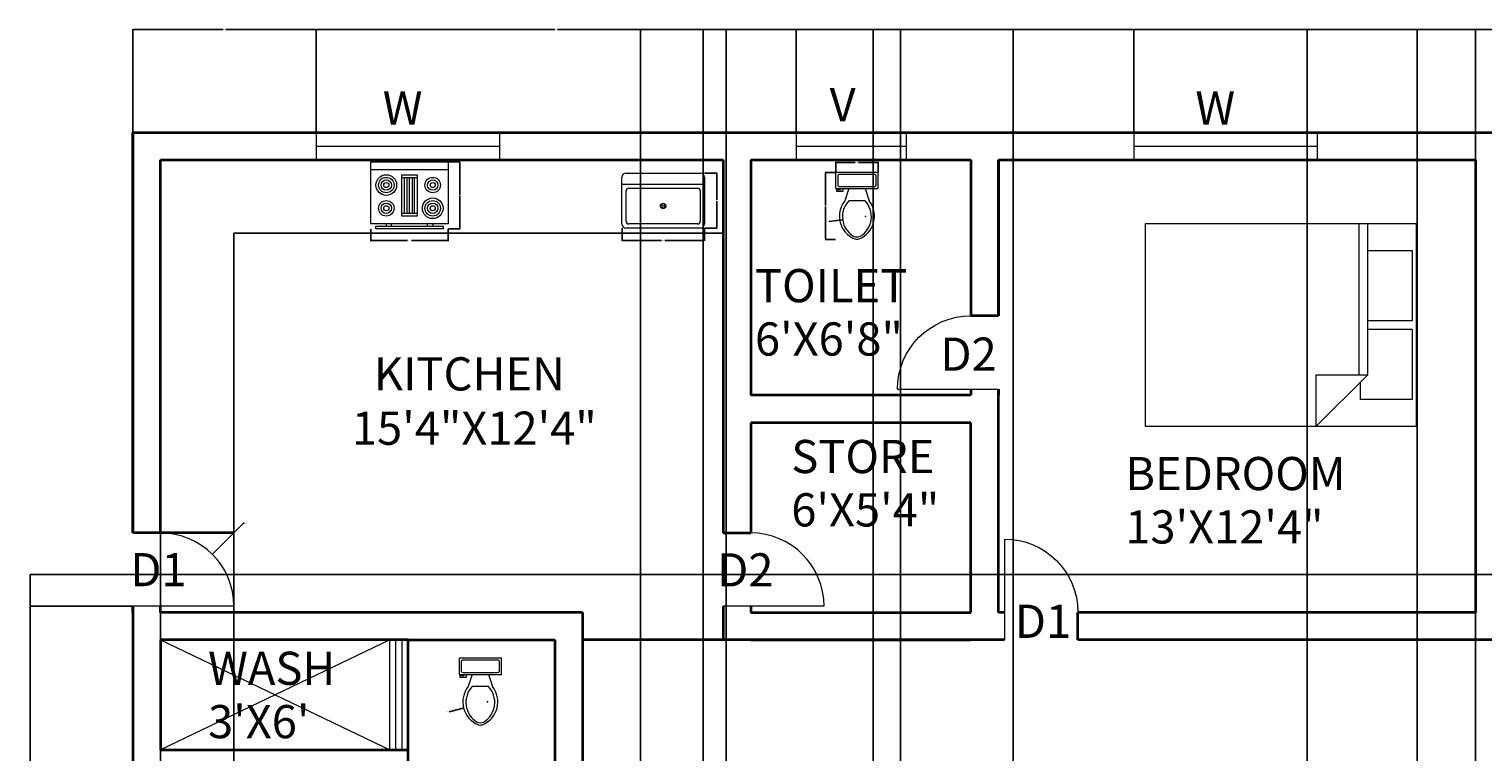
# Model space of a CAD drawing. Units: feet. Extents: x 1681 to 2398, y 1737 to 2411.
# Tile 3 of 4: x 1681 to 2156, y 2174 to 2411. Entities that reach past the tile are written whole.
import ezdxf

# ---------------------------------------------------------------- set-up
doc = ezdxf.new("R2010")
doc.units = ezdxf.units.FT
for name, color, linetype, lineweight in [('A-ANNO-DIMS', 2, 'Continuous', 18), ('A-ANNO-TEXT', 7, 'Continuous', 18), ('A-AREA-IDEN', 7, 'Continuous', 18), ('A-DOOR', 3, 'Continuous', 18), ('A-EQPM', 8, 'Continuous', 18), ('A-FLOR-CASE', 8, 'Continuous', 25), ('A-FLOR-FIXT', 9, 'Continuous', 18), ('A-FURN', 8, 'Continuous', 13), ('A-GLAZ', 4, 'Continuous', 18), ('A-WALL', 7, 'Continuous', 35)]:
    doc.layers.add(name, color=color, linetype=linetype, lineweight=lineweight)
doc.styles.get("Standard").update_dxf_attribs({"font": 'arial.ttf'})
doc.dimstyles.get("Standard").update_dxf_attribs({"dimtxt": 0.18, "dimasz": 0.18, "dimexe": 0.18, "dimexo": 0.0625, "dimgap": 0.09, "dimtad": 0, "dimtih": 1, "dimtoh": 1, "dimdec": 4, "dimzin": 0, "dimdsep": 46, "dimtxsty": 'Standard', "dimcen": 0.09, "dimadec": 0, "dimazin": 0, "dimtfac": 1, "dimtdec": 4, "dimtofl": 0, "dimtmove": 0, "dimatfit": 3, "dimfxl": 1, "dimtolj": 1, "dimtzin": 0, "dimarcsym": 0})

# ---------------------------------------------------------------- blocks, each defined once
blk = doc.blocks.new('Sink-single - 30 in top')
blk.add_line((-15, -3.999996), (15, -3.999996))
for points in [[(-13.5, 0), (13.5, 0)], [(-15, -18.499996), (-15, -1.5)], [(15, -1.5), (15, -18.499996)], [(-13.5, -17.499996), (-13.5, -6.499996)], [(-12.5, -5.499996), (12.5, -5.499996)], [(13.5, -6.499996), (13.5, -17.499996)], [(13.5, -19.999996), (-13.5, -19.999996)], [(12.5, -18.499996), (-12.5, -18.499996)]]:
    blk.add_lwpolyline(points)
for radius in [1, 0.5]:
    blk.add_circle((0, -11.999996), radius)
for centre, radius, start, end in [((-13.5, -1.5), 1.5, 90, 180), ((13.5, -1.5), 1.5, 0, 90), ((-12.5, -6.499996), 1, 90, 180), ((12.5, -6.499996), 1, 0, 90), ((-13.5, -18.499996), 1.5, 180, 270), ((-12.5, -17.499996), 1, 180, 270), ((12.5, -17.499996), 1, 270, 0), ((13.5, -18.499996), 1.5, 270, 0)]:
    blk.add_arc(centre, radius, start, end)
blk = doc.blocks.new('Range-Oven - 30 in top')
for p, q in [((0, -3), (30, -3)), ((12, -6), (18, -6)), ((13, -20), (13, -6)), ((14, -6), (14, -20)), ((15, -20), (15, -6)), ((16, -6), (16, -20)), ((17, -20), (17, -6)), ((18, -20), (12, -20)), ((6, -24), (6, -25)), ((8, -25), (8, -24)), ((22, -25), (22, -24)), ((24, -24), (24, -25))]:
    blk.add_line(p, q)
for points in [[(0, -24), (0, 0), (30, 0), (30, -24)], [(12, -21), (12, -5), (18, -5), (18, -21)], [(2, -26), (2, -25), (28, -25), (28, -26)]]:
    blk.add_lwpolyline(points, close=True)
for centre, radius in [((6, -9), 4), ((6, -9), 3), ((6, -9), 2), ((6, -9), 1), ((24, -9), 3), ((24, -9), 2), ((24, -9), 1), ((6, -18), 3), ((6, -18), 2), ((24, -18), 4), ((24, -18), 3), ((24, -18), 2), ((6, -18), 1), ((24, -18), 1)]:
    blk.add_circle(centre, radius)
blk = doc.blocks.new('Bed - Queen')
for p, q in [((0, -80.00003), (0, 0)), ((0, 0), (59.99999, 0)), ((59.99999, 0), (59.99999, -80.00003)), ((7.99999, -1.2), (28.79998, -1.2)), ((7.99999, -14.4), (7.99999, -1.2)), ((28.79998, -1.2), (28.79998, -14.4)), ((31.19999, -1.2), (51.99999, -1.2)), ((31.19999, -14.4), (31.19999, -1.2)), ((51.99999, -1.2), (51.99999, -16.4)), ((0, -14.4), (44.8, -14.4)), ((44.8, -16.8), (0, -16.8)), ((59.99999, -29.6), (44.8, -14.4)), ((44.8, -14.4), (44.8, -29.6)), ((51.99999, -16.4), (46.79936, -16.4)), ((44.8, -29.6), (59.99999, -29.6)), ((59.99999, -80.00003), (0, -80.00003))]:
    blk.add_line(p, q)
blk = doc.blocks.new('Toilet - top')
for p, q in [((9.5, -6), (9.5, -2)), ((-10, -8.5), (-8, -8.5)), ((-10, -9.5), (-10, -8.5)), ((-7, -9.5), (-10, -9.5)), ((-8, -8.5), (-8, -8)), ((-7, -8), (-7, -9.5)), ((-4, -8), (-6, -14)), ((4, -14), (-4, -14)), ((4, -8), (6, -14))]:
    blk.add_line(p, q)
blk.add_lwpolyline([(10.5, -8), (10.5, 0), (-10.5, 0), (-10.5, -8)], close=True)
for points in [[(-9.5, -2), (-9.5, -6)], [(8.5, -1), (-8.5, -1)], [(-8.5, -7), (8.5, -7)]]:
    blk.add_lwpolyline(points)
for centre, radius, start, end in [((-8.62, -1.88), 0.884, 81.8699, 188.1301), ((-8.62, -6.12), 0.884, 171.8699, 278.1301), ((8.62, -1.88), 0.884, 351.8699, 98.1301), ((8.62, -6.12), 0.884, 261.8699, 8.1301), ((3.52, -21.58), 12.17, 141.46911, 247.97143), ((4.2, -21.82), 11.33, 136.36773, 238.94682), ((-3.52, -21.58), 12.17, 292.02843, 38.53071), ((-4.2, -21.82), 11.33, 301.05301, 43.63209), ((0, -27.88), 4, 245.73182, 294.26817), ((0, -29), 4, 254.86053, 285.13947)]:
    blk.add_arc(centre, radius, start, end)
blk = doc.blocks.new('DOOR-SINGLE-SWING')
blk.add_line((33, 0), (0, 0))
blk.add_arc((9, 0), 24, 0, 90)
blk = doc.blocks.new('WINDOW-STANDARD')
for p, q in [((0, 9), (0, 0)), ((60, 9), (60, 0)), ((0, 4.5), (60, 4.5))]:
    blk.add_line(p, q)
blk = doc.blocks.new('WINDOW-VENTILATOR')
for p, q in [((0, 9), (0, 0)), ((36, 9), (36, 0)), ((0, 4.5), (36, 4.5))]:
    blk.add_line(p, q)
blk = doc.blocks.new('*D20')
at = {"layer": 'A-ANNO-DIMS', "color": 0, "lineweight": -2, "transparency": 16777216}
for p, q in [((1944.47, 2363.95), (1941.06, 2363.95)), ((1941.24, 2363.77), (1941.24, 2353.18)), ((1941.24, 2342.24), (1941.24, 2352.82)), ((1944.47, 2342.06), (1941.06, 2342.06))]:
    blk.add_line(p, q, dxfattribs=at)
at = {"layer": 'A-ANNO-DIMS', "color": 0, "transparency": 16777216}
for points in [[(1941.21, 2363.77), (1941.27, 2363.77), (1941.24, 2363.95)], [(1941.21, 2342.24), (1941.27, 2342.24), (1941.24, 2342.06)]]:
    blk.add_solid(points, dxfattribs=at)
at = {"layer": 'Defpoints', "color": 0, "transparency": 16777216}
for p in [(1941.24, 2363.95), (1944.53, 2363.95), (1944.53, 2342.06)]:
    blk.add_point(p, dxfattribs=at)
at = {"layer": 'A-ANNO-DIMS', "color": 0, "transparency": 16777216, "insert": (1941.24, 2353), "char_height": 0.18, "attachment_point": 5}
blk.add_mtext('\\A1;WC 22 TYP.', dxfattribs=at)
blk = doc.blocks.new('*D21')
at = {"layer": 'A-ANNO-DIMS', "color": 0, "lineweight": -2, "transparency": 16777216}
for p, q in [((1944.53, 2364.01), (1944.53, 2367.41)), ((1944.71, 2367.23), (1950.96, 2367.23)), ((1958.26, 2367.23), (1952, 2367.23)), ((1958.44, 2364.01), (1958.44, 2367.41))]:
    blk.add_line(p, q, dxfattribs=at)
at = {"layer": 'A-ANNO-DIMS', "color": 0, "transparency": 16777216}
for points in [[(1944.71, 2367.26), (1944.71, 2367.2), (1944.53, 2367.23)], [(1958.26, 2367.26), (1958.26, 2367.2), (1958.44, 2367.23)]]:
    blk.add_solid(points, dxfattribs=at)
at = {"layer": 'Defpoints', "color": 0, "transparency": 16777216}
for p in [(1944.53, 2363.95), (1958.44, 2367.23), (1958.44, 2363.95)]:
    blk.add_point(p, dxfattribs=at)
at = {"layer": 'A-ANNO-DIMS', "color": 0, "transparency": 16777216, "insert": (1951.48, 2367.23), "char_height": 0.18, "attachment_point": 5}
blk.add_mtext('\\A1;14 TYP.', dxfattribs=at)
blk = doc.blocks.new('*D32')
at = {"layer": 'A-ANNO-DIMS', "color": 0, "lineweight": -2, "transparency": 16777216}
for p, q in [((1874.66, 2345.7), (1874.66, 2341.54)), ((1901.6, 2345.7), (1901.6, 2341.54)), ((1874.84, 2341.72), (1887.58, 2341.72)), ((1901.42, 2341.72), (1888.68, 2341.72))]:
    blk.add_line(p, q, dxfattribs=at)
at = {"layer": 'A-ANNO-DIMS', "color": 0, "transparency": 16777216}
for points in [[(1874.84, 2341.75), (1874.84, 2341.69), (1874.66, 2341.72)], [(1901.42, 2341.75), (1901.42, 2341.69), (1901.6, 2341.72)]]:
    blk.add_solid(points, dxfattribs=at)
at = {"layer": 'Defpoints', "color": 0, "transparency": 16777216}
for p in [(1874.66, 2345.76), (1901.6, 2345.76), (1901.6, 2341.72)]:
    blk.add_point(p, dxfattribs=at)
at = {"layer": 'A-ANNO-DIMS', "color": 0, "transparency": 16777216, "insert": (1888.13, 2341.72), "char_height": 0.18, "attachment_point": 5}
blk.add_mtext('\\A1;SINK 27', dxfattribs=at)
blk = doc.blocks.new('*D33')
at = {"layer": 'A-ANNO-DIMS', "color": 0, "lineweight": -2, "transparency": 16777216}
for p, q in [((1901.67, 2363.73), (1905.82, 2363.73)), ((1905.64, 2363.55), (1905.64, 2354.93)), ((1905.64, 2345.94), (1905.64, 2354.56)), ((1901.67, 2345.76), (1905.82, 2345.76))]:
    blk.add_line(p, q, dxfattribs=at)
at = {"layer": 'A-ANNO-DIMS', "color": 0, "transparency": 16777216}
for points in [[(1905.61, 2363.55), (1905.67, 2363.55), (1905.64, 2363.73)], [(1905.61, 2345.94), (1905.67, 2345.94), (1905.64, 2345.76)]]:
    blk.add_solid(points, dxfattribs=at)
at = {"layer": 'Defpoints', "color": 0, "transparency": 16777216}
for p in [(1901.6, 2363.73), (1905.64, 2363.73), (1901.6, 2345.76)]:
    blk.add_point(p, dxfattribs=at)
at = {"layer": 'A-ANNO-DIMS', "color": 0, "transparency": 16777216, "insert": (1905.64, 2354.74), "char_height": 0.18, "attachment_point": 5}
blk.add_mtext('\\A1;18', dxfattribs=at)
blk = doc.blocks.new('*D34')
at = {"layer": 'A-ANNO-DIMS', "color": 0, "lineweight": -2, "transparency": 16777216}
for p, q in [((1792.52, 2345.41), (1792.52, 2341.5)), ((1817.82, 2345.41), (1817.82, 2341.5)), ((1792.7, 2341.68), (1804.47, 2341.68)), ((1817.64, 2341.68), (1805.87, 2341.68))]:
    blk.add_line(p, q, dxfattribs=at)
at = {"layer": 'A-ANNO-DIMS', "color": 0, "transparency": 16777216}
for points in [[(1792.7, 2341.71), (1792.7, 2341.65), (1792.52, 2341.68)], [(1817.64, 2341.71), (1817.64, 2341.65), (1817.82, 2341.68)]]:
    blk.add_solid(points, dxfattribs=at)
at = {"layer": 'Defpoints', "color": 0, "transparency": 16777216}
for p in [(1792.52, 2345.47), (1817.82, 2345.47), (1817.82, 2341.68)]:
    blk.add_point(p, dxfattribs=at)
at = {"layer": 'A-ANNO-DIMS', "color": 0, "transparency": 16777216, "insert": (1805.17, 2341.68), "char_height": 0.18, "attachment_point": 5}
blk.add_mtext('\\A1;RANGE 25', dxfattribs=at)
blk = doc.blocks.new('*D35')
at = {"layer": 'A-ANNO-DIMS', "color": 0, "lineweight": -2, "transparency": 16777216}
for p, q in [((1817.88, 2367.4), (1821.79, 2367.4)), ((1821.61, 2367.22), (1821.61, 2356.62)), ((1821.61, 2345.65), (1821.61, 2356.25)), ((1817.88, 2345.47), (1821.79, 2345.47))]:
    blk.add_line(p, q, dxfattribs=at)
at = {"layer": 'A-ANNO-DIMS', "color": 0, "transparency": 16777216}
for points in [[(1821.58, 2367.22), (1821.64, 2367.22), (1821.61, 2367.4)], [(1821.58, 2345.65), (1821.64, 2345.65), (1821.61, 2345.47)]]:
    blk.add_solid(points, dxfattribs=at)
at = {"layer": 'Defpoints', "color": 0, "transparency": 16777216}
for p in [(1817.82, 2367.4), (1821.61, 2367.4), (1817.82, 2345.47)]:
    blk.add_point(p, dxfattribs=at)
at = {"layer": 'A-ANNO-DIMS', "color": 0, "transparency": 16777216, "insert": (1821.61, 2356.44), "char_height": 0.18, "attachment_point": 5}
blk.add_mtext('\\A1;22', dxfattribs=at)
blk = doc.blocks.new('*D42')
at = {"layer": 'A-ANNO-DIMS', "color": 0, "lineweight": -2, "transparency": 16777216}
for p, q in [((1714.74, 2377.11), (1714.74, 2410.83)), ((1714.92, 2410.65), (1744.28, 2410.65)), ((1774.44, 2410.65), (1745.07, 2410.65)), ((1774.62, 2377.11), (1774.62, 2410.83))]:
    blk.add_line(p, q, dxfattribs=at)
at = {"layer": 'A-ANNO-DIMS', "color": 0, "transparency": 16777216}
for points in [[(1714.92, 2410.68), (1714.92, 2410.62), (1714.74, 2410.65)], [(1774.44, 2410.68), (1774.44, 2410.62), (1774.62, 2410.65)]]:
    blk.add_solid(points, dxfattribs=at)
at = {"layer": 'Defpoints', "color": 0, "transparency": 16777216}
for p in [(1774.62, 2410.65), (1714.74, 2377.05), (1774.62, 2377.05)]:
    blk.add_point(p, dxfattribs=at)
at = {"layer": 'A-ANNO-DIMS', "color": 0, "transparency": 16777216, "insert": (1744.68, 2410.65), "char_height": 0.18, "attachment_point": 5}
blk.add_mtext('\\A1;59.88', dxfattribs=at)
blk = doc.blocks.new('*D43')
at = {"layer": 'A-ANNO-DIMS', "color": 0, "lineweight": -2, "transparency": 16777216}
for p, q in [((1774.62, 2377.11), (1774.62, 2410.83)), ((1774.8, 2410.65), (1852.64, 2410.65)), ((1931.39, 2410.65), (1853.55, 2410.65)), ((1931.57, 2377.11), (1931.57, 2410.83))]:
    blk.add_line(p, q, dxfattribs=at)
at = {"layer": 'A-ANNO-DIMS', "color": 0, "transparency": 16777216}
for points in [[(1774.8, 2410.68), (1774.8, 2410.62), (1774.62, 2410.65)], [(1931.39, 2410.68), (1931.39, 2410.62), (1931.57, 2410.65)]]:
    blk.add_solid(points, dxfattribs=at)
at = {"layer": 'Defpoints', "color": 0, "transparency": 16777216}
for p in [(1931.57, 2410.65), (1774.62, 2377.05), (1931.57, 2377.05)]:
    blk.add_point(p, dxfattribs=at)
at = {"layer": 'A-ANNO-DIMS', "color": 0, "transparency": 16777216, "insert": (1853.09, 2410.65), "char_height": 0.18, "attachment_point": 5}
blk.add_mtext('\\A1;156.95', dxfattribs=at)
blk = doc.blocks.new('*D44')
at = {"layer": 'A-ANNO-DIMS', "color": 0, "lineweight": -2, "transparency": 16777216}
for p, q in [((1931.57, 2377.11), (1931.57, 2410.83)), ((1931.75, 2410.65), (1986.34, 2410.65)), ((2041.85, 2410.65), (1987.26, 2410.65)), ((2042.03, 2377.11), (2042.03, 2410.83))]:
    blk.add_line(p, q, dxfattribs=at)
at = {"layer": 'A-ANNO-DIMS', "color": 0, "transparency": 16777216}
for points in [[(1931.75, 2410.68), (1931.75, 2410.62), (1931.57, 2410.65)], [(2041.85, 2410.68), (2041.85, 2410.62), (2042.03, 2410.65)]]:
    blk.add_solid(points, dxfattribs=at)
at = {"layer": 'Defpoints', "color": 0, "transparency": 16777216}
for p in [(2042.03, 2410.65), (1931.57, 2377.05), (2042.03, 2377.05)]:
    blk.add_point(p, dxfattribs=at)
at = {"layer": 'A-ANNO-DIMS', "color": 0, "transparency": 16777216, "insert": (1986.8, 2410.65), "char_height": 0.18, "attachment_point": 5}
blk.add_mtext('\\A1;110.47', dxfattribs=at)
blk = doc.blocks.new('*D45')
at = {"layer": 'A-ANNO-DIMS', "color": 0, "lineweight": -2, "transparency": 16777216}
for p, q in [((2042.03, 2377.11), (2042.03, 2410.83)), ((2042.21, 2410.65), (2127.5, 2410.65)), ((2213.71, 2410.65), (2128.42, 2410.65)), ((2213.89, 2377.11), (2213.89, 2410.83))]:
    blk.add_line(p, q, dxfattribs=at)
at = {"layer": 'A-ANNO-DIMS', "color": 0, "transparency": 16777216}
for points in [[(2042.21, 2410.68), (2042.21, 2410.62), (2042.03, 2410.65)], [(2213.71, 2410.68), (2213.71, 2410.62), (2213.89, 2410.65)]]:
    blk.add_solid(points, dxfattribs=at)
at = {"layer": 'Defpoints', "color": 0, "transparency": 16777216}
for p in [(2213.89, 2410.65), (2042.03, 2377.05), (2213.89, 2377.05)]:
    blk.add_point(p, dxfattribs=at)
at = {"layer": 'A-ANNO-DIMS', "color": 0, "transparency": 16777216, "insert": (2127.96, 2410.65), "char_height": 0.18, "attachment_point": 5}
blk.add_mtext('\\A1;171.85', dxfattribs=at)
blk = doc.blocks.new('*D49')
at = {"layer": 'A-ANNO-DIMS', "color": 0, "lineweight": -2, "transparency": 16777216}
for p, q in [((1714.68, 2222.05), (1680.96, 2222.05)), ((1681.14, 2221.87), (1681.14, 2170.9)), ((1681.14, 2119.58), (1681.14, 2170.54)), ((1714.68, 2119.4), (1680.96, 2119.4))]:
    blk.add_line(p, q, dxfattribs=at)
at = {"layer": 'A-ANNO-DIMS', "color": 0, "transparency": 16777216}
for points in [[(1681.11, 2221.87), (1681.17, 2221.87), (1681.14, 2222.05)], [(1681.11, 2119.58), (1681.17, 2119.58), (1681.14, 2119.4)]]:
    blk.add_solid(points, dxfattribs=at)
at = {"layer": 'Defpoints', "color": 0, "transparency": 16777216}
for p in [(1681.14, 2222.05), (1714.74, 2222.05), (1714.74, 2119.4)]:
    blk.add_point(p, dxfattribs=at)
at = {"layer": 'A-ANNO-DIMS', "color": 0, "transparency": 16777216, "insert": (1681.14, 2170.72), "char_height": 0.18, "attachment_point": 5}
blk.add_mtext('\\A1;102.65', dxfattribs=at)
blk = doc.blocks.new('*D50')
at = {"layer": 'A-ANNO-DIMS', "color": 0, "lineweight": -2, "transparency": 16777216}
for p, q in [((2330.68, 2232.39), (1680.96, 2232.39)), ((1681.14, 2232.21), (1681.14, 2167.4)), ((1681.14, 2102.23), (1681.14, 2167.04)), ((2330.68, 2102.05), (1680.96, 2102.05))]:
    blk.add_line(p, q, dxfattribs=at)
at = {"layer": 'A-ANNO-DIMS', "color": 0, "transparency": 16777216}
for points in [[(1681.11, 2232.21), (1681.17, 2232.21), (1681.14, 2232.39)], [(1681.11, 2102.23), (1681.17, 2102.23), (1681.14, 2102.05)]]:
    blk.add_solid(points, dxfattribs=at)
at = {"layer": 'Defpoints', "color": 0, "transparency": 16777216}
for p in [(1681.14, 2232.39), (2330.74, 2232.39), (2330.74, 2102.05)]:
    blk.add_point(p, dxfattribs=at)
at = {"layer": 'A-ANNO-DIMS', "color": 0, "transparency": 16777216, "insert": (1681.14, 2167.22), "char_height": 0.18, "attachment_point": 5}
blk.add_mtext('\\A1;130.34', dxfattribs=at)
blk = doc.blocks.new('*D51')
at = {"layer": 'A-ANNO-DIMS', "color": 0, "lineweight": -2, "transparency": 16777216}
for p, q in [((1880.74, 1780.11), (1880.74, 2410.83)), ((1880.92, 2410.65), (1890.66, 2410.65)), ((1901.06, 2410.65), (1891.32, 2410.65)), ((1901.24, 1780.11), (1901.24, 2410.83))]:
    blk.add_line(p, q, dxfattribs=at)
at = {"layer": 'A-ANNO-DIMS', "color": 0, "transparency": 16777216}
for points in [[(1880.92, 2410.68), (1880.92, 2410.62), (1880.74, 2410.65)], [(1901.06, 2410.68), (1901.06, 2410.62), (1901.24, 2410.65)]]:
    blk.add_solid(points, dxfattribs=at)
at = {"layer": 'Defpoints', "color": 0, "transparency": 16777216}
for p in [(1901.24, 2410.65), (1880.74, 1780.05), (1901.24, 1780.05)]:
    blk.add_point(p, dxfattribs=at)
at = {"layer": 'A-ANNO-DIMS', "color": 0, "transparency": 16777216, "insert": (1890.99, 2410.65), "char_height": 0.18, "attachment_point": 5}
blk.add_mtext('\\A1;20.5', dxfattribs=at)
blk = doc.blocks.new('*D52')
at = {"layer": 'A-ANNO-DIMS', "color": 0, "lineweight": -2, "transparency": 16777216}
for p, q in [((1965.74, 1780.11), (1965.74, 2410.83)), ((1965.92, 2410.65), (1983.77, 2410.65)), ((2002.37, 2410.65), (1984.52, 2410.65)), ((2002.55, 1780.11), (2002.55, 2410.83))]:
    blk.add_line(p, q, dxfattribs=at)
at = {"layer": 'A-ANNO-DIMS', "color": 0, "transparency": 16777216}
for points in [[(1965.92, 2410.68), (1965.92, 2410.62), (1965.74, 2410.65)], [(2002.37, 2410.68), (2002.37, 2410.62), (2002.55, 2410.65)]]:
    blk.add_solid(points, dxfattribs=at)
at = {"layer": 'Defpoints', "color": 0, "transparency": 16777216}
for p in [(2002.55, 2410.65), (1965.74, 1780.05), (2002.55, 1780.05)]:
    blk.add_point(p, dxfattribs=at)
at = {"layer": 'A-ANNO-DIMS', "color": 0, "transparency": 16777216, "insert": (1984.15, 2410.65), "char_height": 0.18, "attachment_point": 5}
blk.add_mtext('\\A1;36.81', dxfattribs=at)
blk = doc.blocks.new('*D53')
at = {"layer": 'A-ANNO-DIMS', "color": 0, "lineweight": -2, "transparency": 16777216}
for p, q in [((2098.74, 1816.11), (2098.74, 2410.83)), ((2098.92, 2410.65), (2146.52, 2410.65)), ((2194.56, 2410.65), (2146.96, 2410.65)), ((2194.74, 1816.11), (2194.74, 2410.83))]:
    blk.add_line(p, q, dxfattribs=at)
at = {"layer": 'A-ANNO-DIMS', "color": 0, "transparency": 16777216}
for points in [[(2098.92, 2410.68), (2098.92, 2410.62), (2098.74, 2410.65)], [(2194.56, 2410.68), (2194.56, 2410.62), (2194.74, 2410.65)]]:
    blk.add_solid(points, dxfattribs=at)
at = {"layer": 'Defpoints', "color": 0, "transparency": 16777216}
for p in [(2194.74, 2410.65), (2098.74, 1816.05), (2194.74, 1816.05)]:
    blk.add_point(p, dxfattribs=at)
at = {"layer": 'A-ANNO-DIMS', "color": 0, "transparency": 16777216, "insert": (2146.74, 2410.65), "char_height": 0.18, "attachment_point": 5}
blk.add_mtext('\\A1;96', dxfattribs=at)
blk = doc.blocks.new('*D55')
at = {"layer": 'A-ANNO-DIMS', "color": 0, "lineweight": -2, "transparency": 16777216}
for p, q in [((2098.74, 1896.11), (2098.74, 2410.83)), ((2098.92, 2410.65), (2116.52, 2410.65)), ((2134.56, 2410.65), (2116.96, 2410.65)), ((2134.74, 1896.11), (2134.74, 2410.83))]:
    blk.add_line(p, q, dxfattribs=at)
at = {"layer": 'A-ANNO-DIMS', "color": 0, "transparency": 16777216}
for points in [[(2098.92, 2410.68), (2098.92, 2410.62), (2098.74, 2410.65)], [(2134.56, 2410.68), (2134.56, 2410.62), (2134.74, 2410.65)]]:
    blk.add_solid(points, dxfattribs=at)
at = {"layer": 'Defpoints', "color": 0, "transparency": 16777216}
for p in [(2098.74, 2410.65), (2098.74, 1896.05), (2134.74, 1896.05)]:
    blk.add_point(p, dxfattribs=at)
at = {"layer": 'A-ANNO-DIMS', "color": 0, "transparency": 16777216, "insert": (2116.74, 2410.65), "char_height": 0.18, "attachment_point": 5}
blk.add_mtext('\\A1;36', dxfattribs=at)
blk = doc.blocks.new('*D58')
at = {"layer": 'A-ANNO-DIMS', "color": 0, "lineweight": -2, "transparency": 16777216}
for p, q in [((1908.74, 1932.11), (1908.74, 2410.83)), ((1908.92, 2410.65), (1932.52, 2410.65)), ((1956.56, 2410.65), (1932.96, 2410.65)), ((1956.74, 1932.11), (1956.74, 2410.83))]:
    blk.add_line(p, q, dxfattribs=at)
at = {"layer": 'A-ANNO-DIMS', "color": 0, "transparency": 16777216}
for points in [[(1908.92, 2410.68), (1908.92, 2410.62), (1908.74, 2410.65)], [(1956.56, 2410.68), (1956.56, 2410.62), (1956.74, 2410.65)]]:
    blk.add_solid(points, dxfattribs=at)
at = {"layer": 'Defpoints', "color": 0, "transparency": 16777216}
for p in [(1956.74, 2410.65), (1908.74, 1932.05), (1956.74, 1932.05)]:
    blk.add_point(p, dxfattribs=at)
at = {"layer": 'A-ANNO-DIMS', "color": 0, "transparency": 16777216, "insert": (1932.74, 2410.65), "char_height": 0.18, "attachment_point": 5}
blk.add_mtext('\\A1;48', dxfattribs=at)
blk = doc.blocks.new('*D59')
at = {"layer": 'A-ANNO-DIMS', "color": 0, "lineweight": -2, "transparency": 16777216}
for p, q in [((2098.74, 1941.11), (2098.74, 2410.83)), ((2098.92, 2410.65), (2126.02, 2410.65)), ((2153.56, 2410.65), (2126.46, 2410.65)), ((2153.74, 1941.11), (2153.74, 2410.83))]:
    blk.add_line(p, q, dxfattribs=at)
at = {"layer": 'A-ANNO-DIMS', "color": 0, "transparency": 16777216}
for points in [[(2098.92, 2410.68), (2098.92, 2410.62), (2098.74, 2410.65)], [(2153.56, 2410.68), (2153.56, 2410.62), (2153.74, 2410.65)]]:
    blk.add_solid(points, dxfattribs=at)
at = {"layer": 'Defpoints', "color": 0, "transparency": 16777216}
for p in [(2153.74, 2410.65), (2098.74, 1941.05), (2153.74, 1941.05)]:
    blk.add_point(p, dxfattribs=at)
at = {"layer": 'A-ANNO-DIMS', "color": 0, "transparency": 16777216, "insert": (2126.24, 2410.65), "char_height": 0.18, "attachment_point": 5}
blk.add_mtext('\\A1;55', dxfattribs=at)
blk = doc.blocks.new('*D60')
at = {"layer": 'A-ANNO-DIMS', "color": 0, "lineweight": -2, "transparency": 16777216}
for p, q in [((1723.74, 2245.99), (1723.74, 1737.27)), ((1747.74, 2245.99), (1747.74, 1737.27)), ((1723.92, 1737.45), (1735.52, 1737.45)), ((1747.56, 1737.45), (1735.96, 1737.45))]:
    blk.add_line(p, q, dxfattribs=at)
at = {"layer": 'A-ANNO-DIMS', "color": 0, "transparency": 16777216}
for points in [[(1723.92, 1737.48), (1723.92, 1737.42), (1723.74, 1737.45)], [(1747.56, 1737.48), (1747.56, 1737.42), (1747.74, 1737.45)]]:
    blk.add_solid(points, dxfattribs=at)
at = {"layer": 'Defpoints', "color": 0, "transparency": 16777216}
for p in [(1723.74, 2246.05), (1747.74, 2246.05), (1747.74, 1737.45)]:
    blk.add_point(p, dxfattribs=at)
at = {"layer": 'A-ANNO-DIMS', "color": 0, "transparency": 16777216, "insert": (1735.74, 1737.45), "char_height": 0.18, "attachment_point": 5}
blk.add_mtext('\\A1;24', dxfattribs=at)
blk = doc.blocks.new('*D63')
at = {"layer": 'A-ANNO-DIMS', "color": 0, "lineweight": -2, "transparency": 16777216}
for p, q in [((1750.89, 2249.2), (1740.84, 2239.15)), ((1751.07, 2249.2), (1750.89, 2249.2)), ((1723.65, 2222.05), (1723.83, 2222.05)), ((1723.74, 2221.96), (1723.74, 2222.14))]:
    blk.add_line(p, q, dxfattribs=at)
at = {"layer": 'A-ANNO-DIMS', "color": 0, "transparency": 16777216}
blk.add_solid([(1740.82, 2239.17), (1740.86, 2239.12), (1740.71, 2239.02)], dxfattribs=at)
at = {"layer": 'Defpoints', "color": 0, "transparency": 16777216}
for p in [(1740.71, 2239.02), (1723.74, 2222.05)]:
    blk.add_point(p, dxfattribs=at)
at = {"layer": 'A-ANNO-DIMS', "color": 0, "transparency": 16777216, "insert": (1751.57, 2249.2), "char_height": 0.18, "attachment_point": 5}
blk.add_mtext('\\A1;9X R24', dxfattribs=at)
blk = doc.blocks.new('*D68')
at = {"layer": 'A-ANNO-DIMS', "color": 0, "lineweight": -2, "transparency": 16777216}
for p, q in [((1818.19, 2187.51), (1822.69, 2188.69)), ((1830.57, 2190.78), (1830.75, 2190.78)), ((1830.66, 2190.69), (1830.66, 2190.87))]:
    blk.add_line(p, q, dxfattribs=at)
at = {"layer": 'A-ANNO-DIMS', "color": 0, "transparency": 16777216}
blk.add_solid([(1822.69, 2188.72), (1822.7, 2188.66), (1822.87, 2188.73)], dxfattribs=at)
at = {"layer": 'Defpoints', "color": 0, "transparency": 16777216}
for p in [(1822.87, 2188.73), (1830.66, 2190.78)]:
    blk.add_point(p, dxfattribs=at)
at = {"layer": 'A-ANNO-DIMS', "color": 0, "transparency": 16777216, "insert": (1817.59, 2187.51), "char_height": 0.18, "attachment_point": 5}
blk.add_mtext('\\A1;8X R8.06', dxfattribs=at)
blk = doc.blocks.new('*D69')
at = {"layer": 'A-ANNO-DIMS', "color": 0, "lineweight": -2, "transparency": 16777216}
for p, q in [((1954.18, 2349.49), (1954.36, 2349.49)), ((1954.27, 2349.4), (1954.27, 2349.58)), ((1942.37, 2347.89), (1946.65, 2348.47))]:
    blk.add_line(p, q, dxfattribs=at)
at = {"layer": 'A-ANNO-DIMS', "color": 0, "transparency": 16777216}
blk.add_solid([(1946.65, 2348.5), (1946.65, 2348.44), (1946.83, 2348.49)], dxfattribs=at)
at = {"layer": 'Defpoints', "color": 0, "transparency": 16777216}
for p in [(1954.27, 2349.49), (1946.83, 2348.49)]:
    blk.add_point(p, dxfattribs=at)
at = {"layer": 'A-ANNO-DIMS', "color": 0, "transparency": 16777216, "insert": (1941.69, 2347.89), "char_height": 0.18, "attachment_point": 5}
blk.add_mtext('\\A1;8X R7.504', dxfattribs=at)

msp = doc.modelspace()

# ---------------------------------------------------------------- linework, layer by layer
at = {"layer": 'A-FLOR-CASE'}
for p, q in [((1747.7402, 2344.0485), (1907.7402, 2344.0485)), ((1747.7402, 2246.0485), (1747.7402, 2344.0485))]:
    msp.add_line(p, q, dxfattribs=at)
at = {"layer": 'A-FLOR-FIXT'}
for p, q in [((1723.7402, 2211.0485), (1798.7402, 2175.0485)), ((1798.7402, 2211.0485), (1723.7402, 2175.0485)), ((1798.7402, 2175.0485), (1798.7402, 2211.0485)), ((1800.7402, 2175.0485), (1800.7402, 2211.0485)), ((1802.7402, 2175.0485), (1802.7402, 2211.0485)), ((1798.7402, 2175.0485), (1723.7402, 2175.0485))]:
    msp.add_line(p, q, dxfattribs=at)
at = {"layer": 'A-WALL'}
for p, q in [((1714.7402, 2377.0485), (2339.7402, 2377.0485)), ((1714.7402, 2377.0485), (1714.7402, 2246.0485)), ((1714.7402, 2377.0485), (1714.7402, 2246.0485)), ((1714.7402, 2377.0485), (1714.7402, 2246.0485)), ((1714.7402, 2246.0485), (1714.7402, 2377.0485)), ((1916.7402, 2377.0485), (2339.7402, 2377.0485)), ((1997.7402, 2377.0485), (2153.7402, 2377.0485)), ((1723.7402, 2368.0485), (1907.7402, 2368.0485)), ((1723.7402, 2246.0485), (1723.7402, 2368.0485)), ((1907.7402, 2368.0485), (1907.7402, 2246.0485)), ((1916.7402, 2368.0485), (1916.7402, 2291.0485)), ((1916.7402, 2368.0485), (1988.7402, 2368.0485)), ((1988.7402, 2368.0485), (1988.7402, 2317.0485)), ((1997.7402, 2368.0485), (1997.7402, 2317.0485)), ((1997.7402, 2368.0485), (2153.7402, 2368.0485)), ((1997.7402, 2317.0485), (1997.7402, 2368.0485)), ((2153.7402, 2368.0485), (2153.7402, 2220.0485)), ((1997.7402, 2317.0485), (1988.7402, 2317.0485)), ((1988.7402, 2293.0485), (1988.7402, 2291.0485)), ((1997.7402, 2220.0485), (1997.7402, 2293.0485)), ((1997.7402, 2293.0485), (1997.7402, 2291.0485)), ((1988.7402, 2291.0485), (1916.7402, 2291.0485)), ((1988.7402, 2282.0485), (1916.7402, 2282.0485)), ((1916.7402, 2282.0485), (1916.7402, 2246.0485)), ((1988.7402, 2220.0485), (1988.7402, 2282.0485)), ((1747.7402, 2246.0485), (1714.7402, 2246.0485)), ((1907.7402, 2246.0485), (1916.7402, 2246.0485)), ((1714.7402, 2220.0485), (1714.7402, 2222.0485)), ((1714.7402, 2222.0485), (1714.7402, 2102.0485)), ((1714.7402, 2222.0485), (1714.7402, 2175.0485)), ((1714.7402, 2222.0485), (1714.7402, 1771.0485)), ((1723.7402, 2220.0485), (1723.7402, 2222.0485)), ((1907.7402, 2222.0485), (1907.7402, 2211.0485)), ((1916.7402, 2222.0485), (1916.7402, 2220.0485)), ((1861.7402, 2220.0485), (1723.7402, 2220.0485)), ((1861.7402, 2220.0485), (1861.7402, 2128.0485)), ((1916.7402, 2220.0485), (1988.7402, 2220.0485)), ((1999.7402, 2220.0485), (1997.7402, 2220.0485)), ((2153.7402, 2220.0485), (2023.7402, 2220.0485)), ((2023.7402, 2211.0485), (2023.7402, 2220.0485)), ((1723.7402, 2211.0485), (1723.7402, 2175.0485)), ((1804.7402, 2211.0485), (1723.7402, 2211.0485)), ((1804.7402, 2175.0485), (1804.7402, 2211.0485)), ((1804.7402, 2102.0485), (1804.7402, 2211.0485)), ((1804.7402, 2211.0485), (1852.7402, 2211.0485)), ((1852.7402, 2211.0485), (1852.7402, 2128.0485)), ((1999.7402, 2211.0485), (1861.7402, 2211.0485)), ((1916.7402, 2211.0485), (1988.7402, 2211.0485)), ((2162.7402, 2211.0485), (2023.7402, 2211.0485)), ((1723.7402, 2175.0485), (1804.7402, 2175.0485))]:
    msp.add_line(p, q, dxfattribs=at)

# ---------------------------------------------------------------- block references
at = {"layer": 'A-DOOR', "extrusion": (0, 0, -1), "zscale": -1}
msp.add_blockref('DOOR-SINGLE-SWING', (-1997.7402, 2293.0485), dxfattribs=at)
at = {"layer": 'A-DOOR'}
for p in [(1714.7402, 2222.0485), (1907.7402, 2222.0485)]:
    msp.add_blockref('DOOR-SINGLE-SWING', p, dxfattribs=at)
at = {"layer": 'A-DOOR', "extrusion": (0, 0, -1), "zscale": -1, "rotation": 90.00000000000003}
msp.add_blockref('DOOR-SINGLE-SWING', (-1999.7402, 2211.0485), dxfattribs=at)
at = {"layer": 'A-EQPM', "xscale": 0.8432003665190245, "yscale": 0.8432003665190245, "zscale": 0.8432003665190245}
msp.add_blockref('Range-Oven - 30 in top', (1792.5218, 2367.3969), dxfattribs=at)
at = {"layer": 'A-FLOR-FIXT'}
for name, p, xscale, yscale, zscale in [('Sink-single - 30 in top', (1888.1298, 2363.727), 0.8982043116384206, 0.8982043116384206, 0.8982043116384206), ('Toilet - top', (1951.4831, 2363.9453), 0.6624009790136799, 0.6624009790136799, 0.6624009790136799), ('Toilet - top', (1828.3332, 2205.0771), 0.6624009790136799, 0.6624009790136799, 0.6624009790136799)]:
    msp.add_blockref(name, p, dxfattribs=dict(at, xscale=xscale, yscale=yscale, zscale=zscale))
at = {"layer": 'A-FURN', "xscale": 1.106801235632363, "yscale": 1.106801235632363, "zscale": 1.106801235632363, "rotation": 270}
msp.add_blockref('Bed - Queen', (2134.3388, 2347.2426), dxfattribs=at)
at = {"layer": 'A-GLAZ'}
for name, p in [('WINDOW-STANDARD', (1774.6173, 2368.0485)), ('WINDOW-VENTILATOR', (1931.5651, 2368.0485)), ('WINDOW-STANDARD', (2042.0348, 2368.0485))]:
    msp.add_blockref(name, p, dxfattribs=at)

# ---------------------------------------------------------------- texts
at = {"layer": 'A-ANNO-TEXT'}
for s, height, p in [('V', 10.8568, (1942.5443, 2380.7028)), ('W', 10.8568, (1796.4106, 2379.6151)), ('W', 10.8568, (2062.1484, 2379.6079)), ('D2', 10.85679, (1978.7815, 2299.0839)), ('D1', 10.85679, (1713.8691, 2228.5946)), ('D2', 10.85679, (1905.7813, 2228.5303)), ('D1', 10.85679, (2003.1144, 2211.7121))]:
    msp.add_text(s, height=height, dxfattribs=at).set_placement(p)
at = {"layer": 'A-AREA-IDEN'}
for s, height, p in [('TOILET', 10.85679, (1918.1298, 2321.4834)), ('6\'X6\'8"', 10.85679, (1918.1298, 2304.0429)), ('KITCHEN', 10.85679, (1793.5243, 2292.634)), ('15\'4"X12\'4"', 10.856786, (1786.3344, 2274.8742)), ('STORE', 10.85679, (1930.0149, 2265.5996)), ('BEDROOM', 10.85679, (2039.2337, 2260.0259)), ('6\'X5\'4"', 10.85679, (1930.0149, 2248.1591)), ('13\'X12\'4"', 10.85679, (2039.2337, 2242.5854)), ('WASH', 10.85679, (1739.302, 2196.3382)), ("3'X6'", 10.85679, (1739.302, 2178.8977))]:
    msp.add_text(s, height=height, dxfattribs=at).set_placement(p)

# ---------------------------------------------------------------- dimensions: what is measured, and where the dimension line sits
at = {"layer": 'A-ANNO-DIMS'}
for base, p1, p2, override, picture, middle in [((1774.6173, 2410.6485), (1714.7402, 2377.0485), (1774.6173, 2377.0485), {"dimdec": 2, "dimlfac": 1, "dimrnd": 0, "dimzin": 0, "dimdsep": 46, "dimlunit": 2}, '*D42', (1744.6787, 2410.6485)), ((1931.5651, 2410.6485), (1774.6173, 2377.0485), (1931.5651, 2377.0485), {"dimdec": 2, "dimlfac": 1, "dimrnd": 0, "dimzin": 0, "dimdsep": 46, "dimlunit": 2}, '*D43', (1853.0912, 2410.6485)), ((1901.2406, 2410.6485), (1880.7402, 1780.0485), (1901.2406, 1780.0485), {"dimdec": 1, "dimlfac": 1, "dimrnd": 0, "dimzin": 0, "dimdsep": 46, "dimlunit": 2}, '*D51', (1890.9904, 2410.6485)), ((1956.7402, 2410.6485), (1908.7402, 1932.0485), (1956.7402, 1932.0485), {"dimdec": 0, "dimlfac": 1, "dimrnd": 0, "dimzin": 0, "dimdsep": 46, "dimlunit": 2}, '*D58', (1932.7402, 2410.6485)), ((2042.0348, 2410.6485), (1931.5651, 2377.0485), (2042.0348, 2377.0485), {"dimdec": 2, "dimlfac": 1, "dimrnd": 0, "dimzin": 0, "dimdsep": 46, "dimlunit": 2}, '*D44', (1986.7999, 2410.6485)), ((2002.5532, 2410.6485), (1965.7402, 1780.0485), (2002.5532, 1780.0485), {"dimdec": 2, "dimlfac": 1, "dimrnd": 0, "dimzin": 0, "dimdsep": 46, "dimlunit": 2}, '*D52', (1984.1467, 2410.6485)), ((2213.8855, 2410.6485), (2042.0348, 2377.0485), (2213.8855, 2377.0485), {"dimdec": 2, "dimlfac": 1, "dimrnd": 0, "dimzin": 0, "dimdsep": 46, "dimlunit": 2}, '*D45', (2127.9602, 2410.6485)), ((2194.7402, 2410.6485), (2098.7402, 1816.0485), (2194.7402, 1816.0485), {"dimdec": 0, "dimlfac": 1, "dimrnd": 0, "dimzin": 0, "dimdsep": 46, "dimlunit": 2}, '*D53', (2146.7402, 2410.6485)), ((2098.7402, 2410.6485), (2134.7402, 1896.0485), (2098.7402, 1896.0485), {"dimdec": 0, "dimlfac": 1, "dimrnd": 0, "dimzin": 0, "dimdsep": 46, "dimlunit": 2}, '*D55', (2116.7402, 2410.6485)), ((2153.7402, 2410.6485), (2098.7402, 1941.0485), (2153.7402, 1941.0485), {"dimdec": 0, "dimlfac": 1, "dimrnd": 0, "dimzin": 0, "dimdsep": 46, "dimlunit": 2}, '*D59', (2126.2402, 2410.6485)), ((1747.7402, 1737.4485), (1723.7402, 2246.0485), (1747.7402, 2246.0485), {"dimdec": 0, "dimlfac": 1, "dimrnd": 0, "dimzin": 0, "dimdsep": 46, "dimlunit": 2}, '*D60', (1735.7402, 1737.4485))]:
    dim = msp.add_linear_dim(base=base, p1=p1, p2=p2, dimstyle='Standard', override=override, dxfattribs=at)
    dim.commit()
    dim.dimension.update_dxf_attribs({"geometry": picture, "text_midpoint": middle})
for base, p1, p2, override, picture, middle in [((1821.6122, 2367.3969), (1817.8178, 2345.4737), (1817.8178, 2367.3969), {"dimdec": 0, "dimlfac": 1, "dimrnd": 0, "dimzin": 0, "dimdsep": 46, "dimlunit": 2}, '*D35', (1821.6122, 2356.4353)), ((1905.6448, 2363.727), (1901.6028, 2345.7629), (1901.6028, 2363.727), {"dimdec": 0, "dimlfac": 1, "dimrnd": 0, "dimzin": 0, "dimdsep": 46, "dimlunit": 2}, '*D33', (1905.6448, 2354.7449)), ((1681.1402, 2232.3872), (2330.7402, 2102.0485), (2330.7402, 2232.3872), {"dimdec": 2, "dimlfac": 1, "dimrnd": 0, "dimzin": 0, "dimdsep": 46, "dimlunit": 2}, '*D50', (1681.1402, 2167.2178)), ((1681.1402, 2222.0485), (1714.7402, 2119.3956), (1714.7402, 2222.0485), {"dimdec": 2, "dimlfac": 1, "dimrnd": 0, "dimzin": 0, "dimdsep": 46, "dimlunit": 2}, '*D49', (1681.1402, 2170.722))]:
    dim = msp.add_linear_dim(base=base, p1=p1, p2=p2, angle=90, dimstyle='Standard', override=override, dxfattribs=at)
    dim.commit()
    dim.dimension.update_dxf_attribs({"geometry": picture, "text_midpoint": middle})
dim = msp.add_linear_dim(base=(1941.2444, 2363.9453), p1=(1944.5279, 2342.0554), p2=(1944.5279, 2363.9453), angle=90, text='WC <> TYP.', dimstyle='Standard', override={"dimdec": 0, "dimlfac": 1, "dimrnd": 0, "dimzin": 0, "dimdsep": 46, "dimlunit": 2}, dxfattribs=at)
dim.commit()
dim.dimension.update_dxf_attribs({"geometry": '*D20', "text_midpoint": (1941.2444, 2353.0003)})
for base, p1, p2, text, picture, middle in [((1958.4383, 2367.2287), (1944.5279, 2363.9453), (1958.4383, 2363.9453), '<> TYP.', '*D21', (1951.4831, 2367.2287)), ((1817.8178, 2341.6793), (1792.5218, 2345.4737), (1817.8178, 2345.4737), 'RANGE <>', '*D34', (1805.1698, 2341.6793)), ((1901.6028, 2341.721), (1874.6567, 2345.7629), (1901.6028, 2345.7629), 'SINK <>', '*D32', (1888.1298, 2341.721))]:
    dim = msp.add_linear_dim(base=base, p1=p1, p2=p2, text=text, dimstyle='Standard', override={"dimdec": 0, "dimlfac": 1, "dimrnd": 0, "dimzin": 0, "dimdsep": 46, "dimlunit": 2}, dxfattribs=at)
    dim.commit()
    dim.dimension.update_dxf_attribs({"geometry": picture, "text_midpoint": middle})
for center, mpoint, text, override, picture, middle in [((1954.2651, 2349.4934), (1946.8277, 2348.493), '8X <>', {"dimdec": 3, "dimlfac": 1, "dimrnd": 0, "dimzin": 0, "dimdsep": 46, "dimlunit": 2}, '*D69', (1942.3652, 2347.8927)), ((1723.7402, 2222.0485), (1740.7109, 2239.0189), '9X <>', {"dimdec": 0, "dimlfac": 1, "dimrnd": 0, "dimzin": 0, "dimdsep": 46, "dimlunit": 2}, '*D63', (1751.5714, 2249.2011)), ((1830.6645, 2190.7821), (1822.8683, 2188.7341), '8X <>', {"dimdec": 2, "dimlfac": 1, "dimrnd": 0, "dimzin": 0, "dimdsep": 46, "dimlunit": 2}, '*D68', (1818.1905, 2187.5052))]:
    dim = msp.add_radius_dim(center=center, mpoint=mpoint, text=text, dimstyle='Standard', override=override, dxfattribs=at)
    dim.commit()
    dim.dimension.update_dxf_attribs({"geometry": picture, "text_midpoint": middle, "dimtype": 164})

doc.saveas('drawing.dxf')
